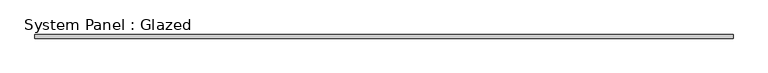
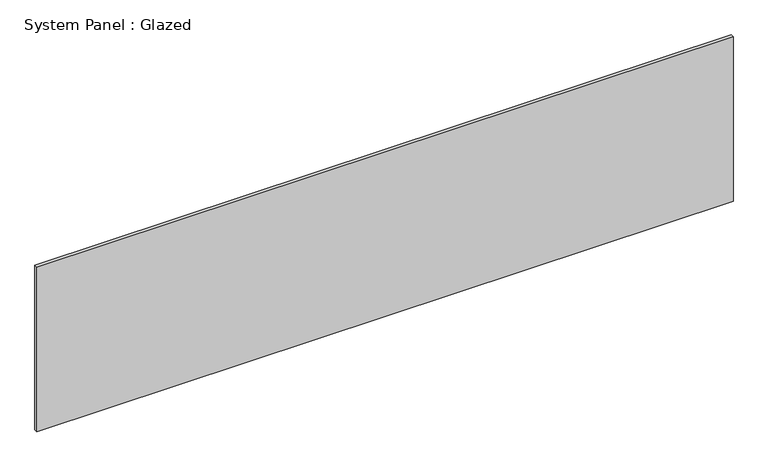
"""IFC4 building model written with IfcOpenShell, lengths in millimetres: plate geometry, System Panel : Glazed."""

from ifc_helpers import new_model, si_unit, origin, origin_with_axes, place, context, project, spatial, polyline, outline, extrude, source, transform, mapped, element, save


def system_panel_glazed_fa2f7082(model_context):
    return source(origin(), model_context, "Body", "SweptSolid", [
        extrude(outline(polyline([(2442.0598823, 19.05), (-2442.0598823, 19.05), (-2442.0598823, 44.45), (2442.0598823, 44.45), (2442.0598823, 19.05)])), origin_with_axes(), (0.0, 0.0, 1.0), 1219.2),
    ])


if __name__ == "__main__":
    model = new_model("IFC4")
    model_context = context("Model", 3, world=origin())
    ifc_project = project(units=[si_unit("LENGTHUNIT", "METRE", prefix="MILLI")], contexts=[model_context])
    site = spatial("IfcSite", under=ifc_project)
    building = spatial("IfcBuilding", under=site)
    placement = place(None, origin())
    system_panel_glazed_shape = system_panel_glazed_fa2f7082(model_context)
    element("IfcPlate", 1, ObjectType="System Panel : Glazed", at=placement, inside=building, context=model_context, shape_type="MappedRepresentation", body=[
        mapped(system_panel_glazed_shape, transform((0.0, 0.0, 0.0), x_axis=(1.0, 0.0, 0.0), y_axis=(0.0, 1.0, 0.0), z_axis=(0.0, 0.0, 1.0))),
    ])
    save(model, "model.ifc")

# Revit data of these elements
# Type "System Panel : Glazed"
#   Construction Type Id = "GSP4R"
#   Analytic Construction = "1/8 in Pilkington single glazing"
#   Visual Light Transmittance = 0.9
#   Solar Heat Gain Coefficient = 0.86
#   Heat Transfer Coefficient (U) = 1.18115 BTU/(h·ft²·°F)
# Element 1 (IfcPlate, "System Panel : Glazed")
#   Materials on its faces: "Glass"
# Materials
#   "Glass": class "Glass", colour RGB 0 128 192, transparency 0.75, Description = "Soda Lime Glass", Cost = 0
